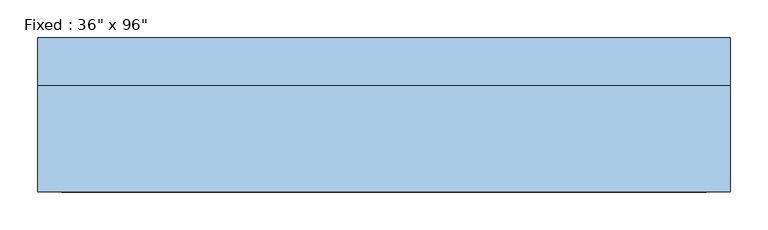
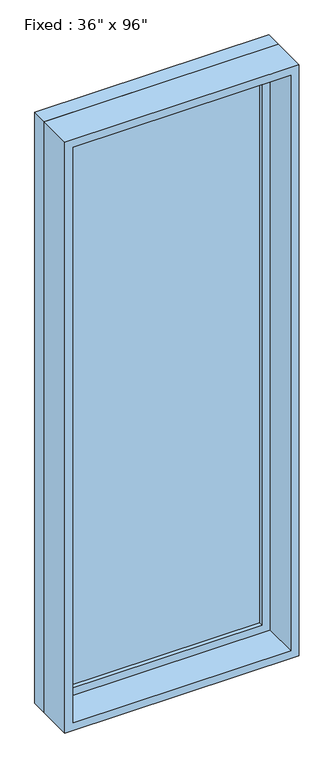
"""IFC4 building model written with IfcOpenShell, lengths in millimetres: window geometry."""

from ifc_helpers import new_model, si_unit, frame, origin, place, context, project, spatial, polyline, outline, extrude, source, transform, mapped, element, save


def window_307ff736(model_context):
    return source(origin(), model_context, "Body", "SweptSolid", [
        extrude(outline(polyline([(355.6, 53.975), (-431.8, 53.975), (-431.8, 66.675), (355.6, 66.675), (355.6, 53.975)])), frame((0.0, 0.0, 368.3), z_axis=(0.0, 0.0, 1.0), x_axis=(1.0, 0.0, 0.0)), (0.0, 0.0, 1.0), 2311.4),
        extrude(outline(polyline([(2724.15, -476.25), (323.85, -476.25), (323.85, 400.05), (2724.15, 400.05), (2724.15, -476.25)]), holes=[polyline([(2679.7, -431.8), (2679.7, 355.6), (368.3, 355.6), (368.3, -431.8), (2679.7, -431.8)])]), frame((0.0, 38.1, 0.0), z_axis=(0.0, 1.0, 0.0), x_axis=(0.0, 0.0, 1.0)), (0.0, 0.0, 1.0), 44.45),
        extrude(outline(polyline([(2743.2, -495.3), (304.8, -495.3), (304.8, 419.1), (2743.2, 419.1), (2743.2, -495.3)]), holes=[polyline([(2711.45, -463.55), (2711.45, 387.35), (336.55, 387.35), (336.55, -463.55), (2711.45, -463.55)])]), frame((0.0, -101.6, 0.0), z_axis=(0.0, 1.0, 0.0), x_axis=(0.0, 0.0, 1.0)), (0.0, 0.0, 1.0), 139.7),
        extrude(outline(polyline([(2743.2, 419.1), (2743.2, -495.3), (304.8, -495.3), (304.8, 419.1), (2743.2, 419.1)]), holes=[polyline([(2724.15, 400.05), (323.85, 400.05), (323.85, -476.25), (2724.15, -476.25), (2724.15, 400.05)])]), frame((0.0, 38.1, 0.0), z_axis=(0.0, 1.0, 0.0), x_axis=(0.0, 0.0, 1.0)), (0.0, 0.0, 1.0), 63.5),
    ])


if __name__ == "__main__":
    model = new_model("IFC4")
    model_context = context("Model", 3, world=origin())
    ifc_project = project(units=[si_unit("LENGTHUNIT", "METRE", prefix="MILLI")], contexts=[model_context])
    site = spatial("IfcSite", under=ifc_project)
    building = spatial("IfcBuilding", under=site)
    placement = place(None, origin())
    window_shape = window_307ff736(model_context)
    element("IfcWindow", 1, ObjectType="Fixed : 36\" x 96\"", at=placement, inside=building, context=model_context, shape_type="MappedRepresentation", body=[
        mapped(window_shape, transform((0.0, 0.0, 0.0), x_axis=(1.0, 0.0, 0.0), y_axis=(0.0, 1.0, 0.0), z_axis=(0.0, 0.0, 1.0))),
    ])
    save(model, "model.ifc")

# Revit data of these elements
# Type "Fixed : 36\" x 96\""
#   Type Mark = "9"
#   Construction Type Id = "GSP4R"
#   Assembly Code = "B2020100"
#   Analytic Construction = "1/8 in Pilkington single glazing"
#   Visual Light Transmittance = 0.9
#   Solar Heat Gain Coefficient = 0.78
#   Heat Transfer Coefficient (U) = 0.6496 BTU/(h·ft²·°F)
#   Height = 8' - 0"
#   Default Sill Height = 1' - 0"
#   Width = 3' - 0"
#   Window Inset = 0' - 0 3/4"
#   Define Thermal Properties by = 1
#   Glass Pane Material = Glass
#   Sash Material = Iron, Ductile
#   Wall Closure = (empty or 0)
# Element 1 (IfcWindow, "Fixed : 36\" x 96\"")
#   Materials on its faces: "Iron, Ductile", "Glass"
# Materials
#   "Glass": class "Glass", colour RGB 0 128 192, transparency 0.75, Description = "Soda Lime Glass", Cost = 0
#   "Iron, Ductile": class "Metal", colour RGB 0 0 0, transparency 0, Description = "Ductile cast iron", Cost = 0
